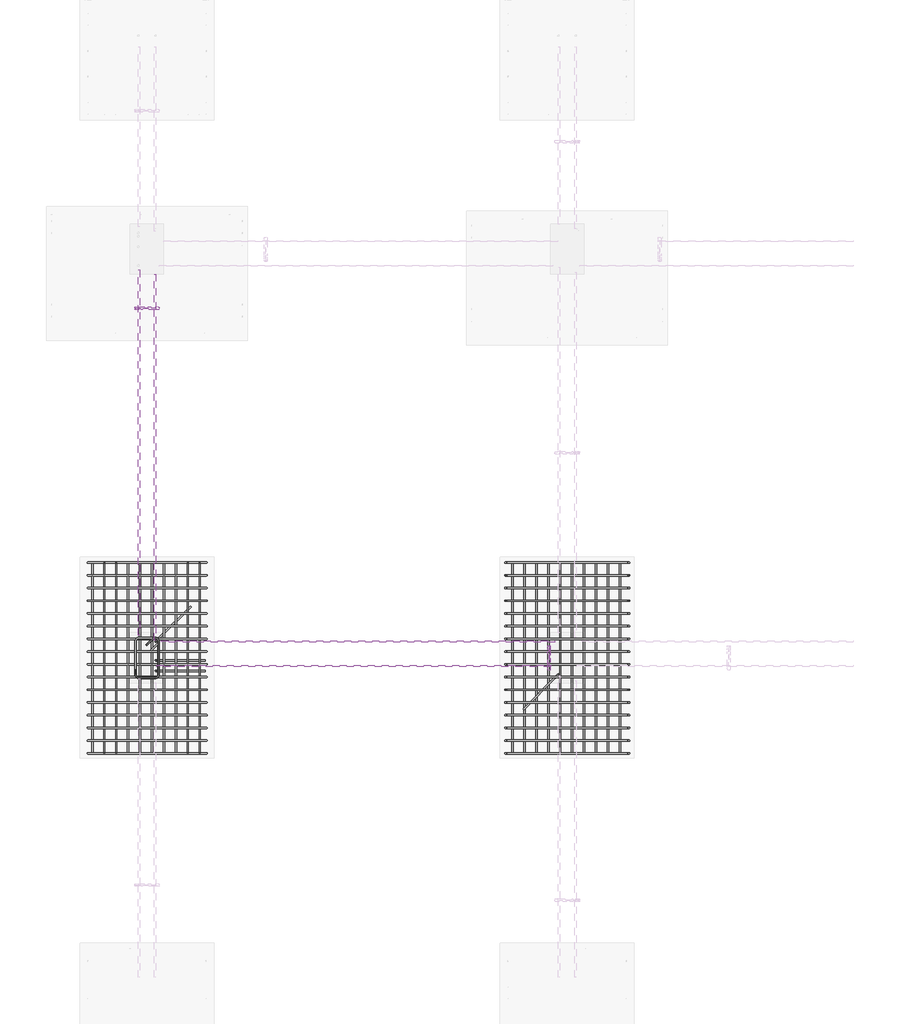
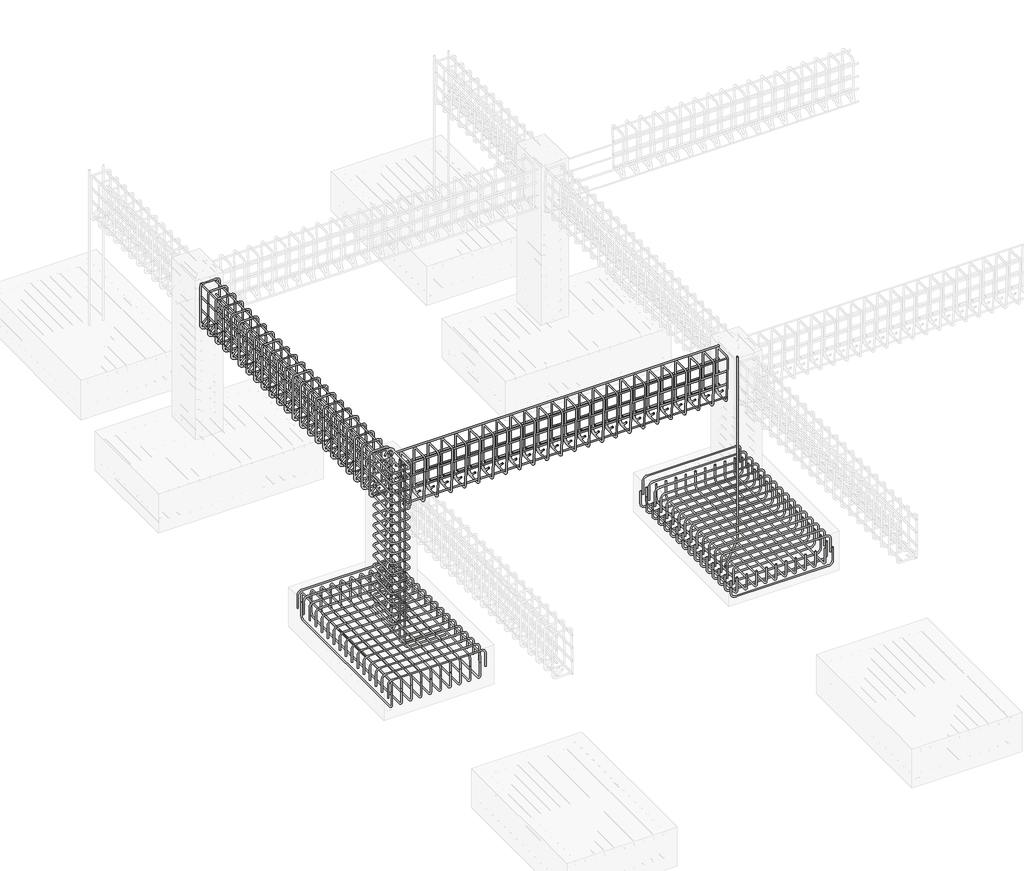
# One storey, part 4 of 20: 16 reinforcing bars.
"""IFC4 building model written with IfcOpenShell, lengths in millimetres."""

from ifc_helpers import new_model, si_unit, point, frame, origin, place, context, project, spatial, polyline, circle_curve, trimmed, segment, composite_curve, source, transform, mapped, element, save
from ifc_brep_helpers import swept_disk

model = new_model("IFC4")

# Units and contexts
model_context = context("Model", 3, world=origin())
ifc_project = project(units=[si_unit("LENGTHUNIT", "METRE", prefix="MILLI")], contexts=[model_context])

# Site, building, storey
site = spatial("IfcSite", under=ifc_project)
building = spatial("IfcBuilding", under=site)
storey = spatial("IfcBuildingStorey", under=building, Elevation=-1828.8)

# Reinforcing bars
placement = place(None, origin())
reinforcing_bar_shape = source(origin(), model_context, "Body", "SolidModel", [
    swept_disk(composite_curve([segment(polyline([(-6393.4168788, -1871.0168637, -2068.8), (-6393.4168788, -1871.0168637, -1921.5)]), True, "CONTINUOUS"), segment(trimmed(circle_curve(frame((-6347.0668788, -1871.0168637, -1921.5), z_axis=(0.0, 1.0, 0.0), x_axis=(-46.349999999999454, 0.0, 0.0)), 46.35), [point((-6393.4168788, -1871.0168637, -1921.5))], [point((-6347.0668788, -1871.0168637, -1875.15))], True, "CARTESIAN"), True, "CONTINUOUS"), segment(polyline([(-6347.0668788, -1871.0168637, -1875.15), (-5379.345487, -1871.0168637, -1875.15)]), True, "CONTINUOUS"), segment(trimmed(circle_curve(frame((-5379.345487, -1871.0168637, -1921.5), z_axis=(0.0, 1.0, 0.0), x_axis=(0.0, 0.0, 46.34999999999991)), 46.35), [point((-5379.345487, -1871.0168637, -1875.15))], [point((-5332.995487, -1871.0168637, -1921.5))], True, "CARTESIAN"), True, "CONTINUOUS"), segment(polyline([(-5332.995487, -1871.0168637, -1921.5), (-5332.995487, -1871.0168637, -2068.8)]), True, "CONTINUOUS")], self_intersect=False), 6.35),
])
element("IfcReinforcingBar", 1, at=placement, inside=storey, context=model_context, shape_type="MappedRepresentation", body=[
    mapped(reinforcing_bar_shape, transform((0.0, 0.0, 0.0), x_axis=(1.0, 0.0, 0.0), y_axis=(0.0, 1.0, 0.0), z_axis=(0.0, 0.0, 1.0))),
    mapped(reinforcing_bar_shape, transform((0.0, -113.82, 0.0), x_axis=(1.0, 0.0, 0.0), y_axis=(0.0, 1.0, 0.0), z_axis=(0.0, 0.0, 1.0))),
    mapped(reinforcing_bar_shape, transform((0.0, -227.64, 0.0), x_axis=(1.0, 0.0, 0.0), y_axis=(0.0, 1.0, 0.0), z_axis=(0.0, 0.0, 1.0))),
    mapped(reinforcing_bar_shape, transform((0.0, -341.46, 0.0), x_axis=(1.0, 0.0, 0.0), y_axis=(0.0, 1.0, 0.0), z_axis=(0.0, 0.0, 1.0))),
    mapped(reinforcing_bar_shape, transform((0.0, -455.28, 0.0), x_axis=(1.0, 0.0, 0.0), y_axis=(0.0, 1.0, 0.0), z_axis=(0.0, 0.0, 1.0))),
    mapped(reinforcing_bar_shape, transform((0.0, -569.1, 0.0), x_axis=(1.0, 0.0, 0.0), y_axis=(0.0, 1.0, 0.0), z_axis=(0.0, 0.0, 1.0))),
    mapped(reinforcing_bar_shape, transform((0.0, -682.92, 0.0), x_axis=(1.0, 0.0, 0.0), y_axis=(0.0, 1.0, 0.0), z_axis=(0.0, 0.0, 1.0))),
    mapped(reinforcing_bar_shape, transform((0.0, -796.74, 0.0), x_axis=(1.0, 0.0, 0.0), y_axis=(0.0, 1.0, 0.0), z_axis=(0.0, 0.0, 1.0))),
    mapped(reinforcing_bar_shape, transform((0.0, -910.56, 0.0), x_axis=(1.0, 0.0, 0.0), y_axis=(0.0, 1.0, 0.0), z_axis=(0.0, 0.0, 1.0))),
    mapped(reinforcing_bar_shape, transform((0.0, -1024.38, 0.0), x_axis=(1.0, 0.0, 0.0), y_axis=(0.0, 1.0, 0.0), z_axis=(0.0, 0.0, 1.0))),
    mapped(reinforcing_bar_shape, transform((0.0, -1138.2, 0.0), x_axis=(1.0, 0.0, 0.0), y_axis=(0.0, 1.0, 0.0), z_axis=(0.0, 0.0, 1.0))),
    mapped(reinforcing_bar_shape, transform((0.0, -1252.02, 0.0), x_axis=(1.0, 0.0, 0.0), y_axis=(0.0, 1.0, 0.0), z_axis=(0.0, 0.0, 1.0))),
    mapped(reinforcing_bar_shape, transform((0.0, -1365.84, 0.0), x_axis=(1.0, 0.0, 0.0), y_axis=(0.0, 1.0, 0.0), z_axis=(0.0, 0.0, 1.0))),
    mapped(reinforcing_bar_shape, transform((0.0, -1479.66, 0.0), x_axis=(1.0, 0.0, 0.0), y_axis=(0.0, 1.0, 0.0), z_axis=(0.0, 0.0, 1.0))),
    mapped(reinforcing_bar_shape, transform((0.0, -1593.48, 0.0), x_axis=(1.0, 0.0, 0.0), y_axis=(0.0, 1.0, 0.0), z_axis=(0.0, 0.0, 1.0))),
    mapped(reinforcing_bar_shape, transform((0.0, -1707.3, 0.0), x_axis=(1.0, 0.0, 0.0), y_axis=(0.0, 1.0, 0.0), z_axis=(0.0, 0.0, 1.0))),
])
reinforcing_bar_2_shape = source(origin(), model_context, "Body", "SolidModel", [
    swept_disk(composite_curve([segment(polyline([(-6353.8495286, -1871.0168637, -2008.6504502), (-6353.8495286, -1871.0168637, -2155.9504502)]), True, "CONTINUOUS"), segment(trimmed(circle_curve(frame((-6353.8495286, -1917.3668637, -2155.9504502), z_axis=(-1.0, 0.0, 0.0), x_axis=(0.0, 46.350000000000136, 0.0)), 46.35), [point((-6353.8495286, -1871.0168637, -2155.9504502))], [point((-6353.8495286, -1917.3668637, -2202.3004502))], True, "CARTESIAN"), True, "CONTINUOUS"), segment(polyline([(-6353.8495286, -1917.3668637, -2202.3004502), (-6353.8495286, -3531.9668637, -2202.3004502)]), True, "CONTINUOUS"), segment(trimmed(circle_curve(frame((-6353.8495286, -3531.9668637, -2155.9504502), z_axis=(-1.0, 0.0, 0.0), x_axis=(0.0, 0.0, -46.34999999999991)), 46.35), [point((-6353.8495286, -3531.9668637, -2202.3004502))], [point((-6353.8495286, -3578.3168637, -2155.9504502))], True, "CARTESIAN"), True, "CONTINUOUS"), segment(polyline([(-6353.8495286, -3578.3168637, -2155.9504502), (-6353.8495286, -3578.3168637, -2008.6504502)]), True, "CONTINUOUS")], self_intersect=False), 6.35),
])
element("IfcReinforcingBar", 2, at=placement, inside=storey, context=model_context, shape_type="MappedRepresentation", body=[
    mapped(reinforcing_bar_2_shape, transform((0.0, 0.0, 0.0), x_axis=(1.0, 0.0, 0.0), y_axis=(0.0, 1.0, 0.0), z_axis=(0.0, 0.0, 1.0))),
    mapped(reinforcing_bar_2_shape, transform((106.7711398, 0.0, 0.0), x_axis=(1.0, 0.0, 0.0), y_axis=(0.0, 1.0, 0.0), z_axis=(0.0, 0.0, 1.0))),
    mapped(reinforcing_bar_2_shape, transform((213.5422797, 0.0, 0.0), x_axis=(1.0, 0.0, 0.0), y_axis=(0.0, 1.0, 0.0), z_axis=(0.0, 0.0, 1.0))),
    mapped(reinforcing_bar_2_shape, transform((320.3134195, 0.0, 0.0), x_axis=(1.0, 0.0, 0.0), y_axis=(0.0, 1.0, 0.0), z_axis=(0.0, 0.0, 1.0))),
    mapped(reinforcing_bar_2_shape, transform((427.0845593, 0.0, 0.0), x_axis=(1.0, 0.0, 0.0), y_axis=(0.0, 1.0, 0.0), z_axis=(0.0, 0.0, 1.0))),
    mapped(reinforcing_bar_2_shape, transform((533.8556992, 0.0, 0.0), x_axis=(1.0, 0.0, 0.0), y_axis=(0.0, 1.0, 0.0), z_axis=(0.0, 0.0, 1.0))),
    mapped(reinforcing_bar_2_shape, transform((640.626839, 0.0, 0.0), x_axis=(1.0, 0.0, 0.0), y_axis=(0.0, 1.0, 0.0), z_axis=(0.0, 0.0, 1.0))),
    mapped(reinforcing_bar_2_shape, transform((747.3979788, 0.0, 0.0), x_axis=(1.0, 0.0, 0.0), y_axis=(0.0, 1.0, 0.0), z_axis=(0.0, 0.0, 1.0))),
    mapped(reinforcing_bar_2_shape, transform((854.1691187, 0.0, 0.0), x_axis=(1.0, 0.0, 0.0), y_axis=(0.0, 1.0, 0.0), z_axis=(0.0, 0.0, 1.0))),
    mapped(reinforcing_bar_2_shape, transform((960.9402585, 0.0, 0.0), x_axis=(1.0, 0.0, 0.0), y_axis=(0.0, 1.0, 0.0), z_axis=(0.0, 0.0, 1.0))),
])
reinforcing_bar_3_shape = source(origin(), model_context, "Body", "SolidModel", [
    swept_disk(composite_curve([segment(polyline([(-5392.9092701, -1871.0168637, -2088.5147466), (-5392.9092701, -1871.0168637, -1941.2147466)]), True, "CONTINUOUS"), segment(trimmed(circle_curve(frame((-5392.9092701, -1917.3668637, -1941.2147466), z_axis=(1.0, 0.0, 0.0), x_axis=(0.0, 46.350000000000136, 0.0)), 46.35), [point((-5392.9092701, -1871.0168637, -1941.2147466))], [point((-5392.9092701, -1917.3668637, -1894.8647466))], True, "CARTESIAN"), True, "CONTINUOUS"), segment(polyline([(-5392.9092701, -1917.3668637, -1894.8647466), (-5392.9092701, -3531.9668637, -1894.8647466)]), True, "CONTINUOUS"), segment(trimmed(circle_curve(frame((-5392.9092701, -3531.9668637, -1941.2147466), z_axis=(1.0, 0.0, 0.0), x_axis=(0.0, 0.0, 46.34999999999991)), 46.35), [point((-5392.9092701, -3531.9668637, -1894.8647466))], [point((-5392.9092701, -3578.3168637, -1941.2147466))], True, "CARTESIAN"), True, "CONTINUOUS"), segment(polyline([(-5392.9092701, -3578.3168637, -1941.2147466), (-5392.9092701, -3578.3168637, -2088.5147466)]), True, "CONTINUOUS")], self_intersect=False), 6.35),
])
element("IfcReinforcingBar", 3, at=placement, inside=storey, context=model_context, shape_type="MappedRepresentation", body=[
    mapped(reinforcing_bar_3_shape, transform((0.0, 0.0, 0.0), x_axis=(1.0, 0.0, 0.0), y_axis=(0.0, 1.0, 0.0), z_axis=(0.0, 0.0, 1.0))),
    mapped(reinforcing_bar_3_shape, transform((-106.7711398, 0.0, 0.0), x_axis=(1.0, 0.0, 0.0), y_axis=(0.0, 1.0, 0.0), z_axis=(0.0, 0.0, 1.0))),
    mapped(reinforcing_bar_3_shape, transform((-213.5422797, 0.0, 0.0), x_axis=(1.0, 0.0, 0.0), y_axis=(0.0, 1.0, 0.0), z_axis=(0.0, 0.0, 1.0))),
    mapped(reinforcing_bar_3_shape, transform((-320.3134195, 0.0, 0.0), x_axis=(1.0, 0.0, 0.0), y_axis=(0.0, 1.0, 0.0), z_axis=(0.0, 0.0, 1.0))),
    mapped(reinforcing_bar_3_shape, transform((-427.0845593, 0.0, 0.0), x_axis=(1.0, 0.0, 0.0), y_axis=(0.0, 1.0, 0.0), z_axis=(0.0, 0.0, 1.0))),
    mapped(reinforcing_bar_3_shape, transform((-533.8556992, 0.0, 0.0), x_axis=(1.0, 0.0, 0.0), y_axis=(0.0, 1.0, 0.0), z_axis=(0.0, 0.0, 1.0))),
    mapped(reinforcing_bar_3_shape, transform((-640.626839, 0.0, 0.0), x_axis=(1.0, 0.0, 0.0), y_axis=(0.0, 1.0, 0.0), z_axis=(0.0, 0.0, 1.0))),
    mapped(reinforcing_bar_3_shape, transform((-747.3979788, 0.0, 0.0), x_axis=(1.0, 0.0, 0.0), y_axis=(0.0, 1.0, 0.0), z_axis=(0.0, 0.0, 1.0))),
    mapped(reinforcing_bar_3_shape, transform((-854.1691187, 0.0, 0.0), x_axis=(1.0, 0.0, 0.0), y_axis=(0.0, 1.0, 0.0), z_axis=(0.0, 0.0, 1.0))),
    mapped(reinforcing_bar_3_shape, transform((-960.9402585, 0.0, 0.0), x_axis=(1.0, 0.0, 0.0), y_axis=(0.0, 1.0, 0.0), z_axis=(0.0, 0.0, 1.0))),
])
reinforcing_bar_4_shape = source(origin(), model_context, "Body", "SolidModel", [
    swept_disk(composite_curve([segment(polyline([(-1549.1360107, -1871.0168637, -2028.4704493), (-1549.1360107, -1871.0168637, -2175.7704493)]), True, "CONTINUOUS"), segment(trimmed(circle_curve(frame((-1595.4860107, -1871.0168637, -2175.7704493), z_axis=(0.0, 1.0, 0.0), x_axis=(46.34999999999991, 0.0, 0.0)), 46.35), [point((-1549.1360107, -1871.0168637, -2175.7704493))], [point((-1595.4860107, -1871.0168637, -2222.1204493))], True, "CARTESIAN"), True, "CONTINUOUS"), segment(polyline([(-1595.4860107, -1871.0168637, -2222.1204493), (-2610.0860107, -1871.0168637, -2222.1204493)]), True, "CONTINUOUS"), segment(trimmed(circle_curve(frame((-2610.0860107, -1871.0168637, -2175.7704493), z_axis=(0.0, 1.0, 0.0), x_axis=(0.0, 0.0, -46.34999999999991)), 46.35), [point((-2610.0860107, -1871.0168637, -2222.1204493))], [point((-2656.4360107, -1871.0168637, -2175.7704493))], True, "CARTESIAN"), True, "CONTINUOUS"), segment(polyline([(-2656.4360107, -1871.0168637, -2175.7704493), (-2656.4360107, -1871.0168637, -2028.4704493)]), True, "CONTINUOUS")], self_intersect=False), 6.35),
])
element("IfcReinforcingBar", 4, at=placement, inside=storey, context=model_context, shape_type="MappedRepresentation", body=[
    mapped(reinforcing_bar_4_shape, transform((0.0, 0.0, 0.0), x_axis=(1.0, 0.0, 0.0), y_axis=(0.0, 1.0, 0.0), z_axis=(0.0, 0.0, 1.0))),
    mapped(reinforcing_bar_4_shape, transform((0.0, -113.82, 0.0), x_axis=(1.0, 0.0, 0.0), y_axis=(0.0, 1.0, 0.0), z_axis=(0.0, 0.0, 1.0))),
    mapped(reinforcing_bar_4_shape, transform((0.0, -227.64, 0.0), x_axis=(1.0, 0.0, 0.0), y_axis=(0.0, 1.0, 0.0), z_axis=(0.0, 0.0, 1.0))),
    mapped(reinforcing_bar_4_shape, transform((0.0, -341.46, 0.0), x_axis=(1.0, 0.0, 0.0), y_axis=(0.0, 1.0, 0.0), z_axis=(0.0, 0.0, 1.0))),
    mapped(reinforcing_bar_4_shape, transform((0.0, -455.28, 0.0), x_axis=(1.0, 0.0, 0.0), y_axis=(0.0, 1.0, 0.0), z_axis=(0.0, 0.0, 1.0))),
    mapped(reinforcing_bar_4_shape, transform((0.0, -569.1, 0.0), x_axis=(1.0, 0.0, 0.0), y_axis=(0.0, 1.0, 0.0), z_axis=(0.0, 0.0, 1.0))),
    mapped(reinforcing_bar_4_shape, transform((0.0, -682.92, 0.0), x_axis=(1.0, 0.0, 0.0), y_axis=(0.0, 1.0, 0.0), z_axis=(0.0, 0.0, 1.0))),
    mapped(reinforcing_bar_4_shape, transform((0.0, -796.74, 0.0), x_axis=(1.0, 0.0, 0.0), y_axis=(0.0, 1.0, 0.0), z_axis=(0.0, 0.0, 1.0))),
    mapped(reinforcing_bar_4_shape, transform((0.0, -910.56, 0.0), x_axis=(1.0, 0.0, 0.0), y_axis=(0.0, 1.0, 0.0), z_axis=(0.0, 0.0, 1.0))),
    mapped(reinforcing_bar_4_shape, transform((0.0, -1024.38, 0.0), x_axis=(1.0, 0.0, 0.0), y_axis=(0.0, 1.0, 0.0), z_axis=(0.0, 0.0, 1.0))),
    mapped(reinforcing_bar_4_shape, transform((0.0, -1138.2, 0.0), x_axis=(1.0, 0.0, 0.0), y_axis=(0.0, 1.0, 0.0), z_axis=(0.0, 0.0, 1.0))),
    mapped(reinforcing_bar_4_shape, transform((0.0, -1252.02, 0.0), x_axis=(1.0, 0.0, 0.0), y_axis=(0.0, 1.0, 0.0), z_axis=(0.0, 0.0, 1.0))),
    mapped(reinforcing_bar_4_shape, transform((0.0, -1365.84, 0.0), x_axis=(1.0, 0.0, 0.0), y_axis=(0.0, 1.0, 0.0), z_axis=(0.0, 0.0, 1.0))),
    mapped(reinforcing_bar_4_shape, transform((0.0, -1479.66, 0.0), x_axis=(1.0, 0.0, 0.0), y_axis=(0.0, 1.0, 0.0), z_axis=(0.0, 0.0, 1.0))),
    mapped(reinforcing_bar_4_shape, transform((0.0, -1593.48, 0.0), x_axis=(1.0, 0.0, 0.0), y_axis=(0.0, 1.0, 0.0), z_axis=(0.0, 0.0, 1.0))),
    mapped(reinforcing_bar_4_shape, transform((0.0, -1707.3, 0.0), x_axis=(1.0, 0.0, 0.0), y_axis=(0.0, 1.0, 0.0), z_axis=(0.0, 0.0, 1.0))),
])
reinforcing_bar_5_shape = source(origin(), model_context, "Body", "SolidModel", [
    swept_disk(composite_curve([segment(polyline([(-2632.2616658, -1871.0168637, -2068.8), (-2632.2616658, -1871.0168637, -1921.5)]), True, "CONTINUOUS"), segment(trimmed(circle_curve(frame((-2585.9116658, -1871.0168637, -1921.5), z_axis=(0.0, 1.0, 0.0), x_axis=(-46.350000000000364, 0.0, 0.0)), 46.35), [point((-2632.2616658, -1871.0168637, -1921.5))], [point((-2585.9116658, -1871.0168637, -1875.15))], True, "CARTESIAN"), True, "CONTINUOUS"), segment(polyline([(-2585.9116658, -1871.0168637, -1875.15), (-1618.1902741, -1871.0168637, -1875.15)]), True, "CONTINUOUS"), segment(trimmed(circle_curve(frame((-1618.1902741, -1871.0168637, -1921.5), z_axis=(0.0, 1.0, 0.0), x_axis=(0.0, 0.0, 46.34999999999991)), 46.35), [point((-1618.1902741, -1871.0168637, -1875.15))], [point((-1571.8402741, -1871.0168637, -1921.5))], True, "CARTESIAN"), True, "CONTINUOUS"), segment(polyline([(-1571.8402741, -1871.0168637, -1921.5), (-1571.8402741, -1871.0168637, -2068.8)]), True, "CONTINUOUS")], self_intersect=False), 6.35),
])
element("IfcReinforcingBar", 5, at=placement, inside=storey, context=model_context, shape_type="MappedRepresentation", body=[
    mapped(reinforcing_bar_5_shape, transform((0.0, 0.0, 0.0), x_axis=(1.0, 0.0, 0.0), y_axis=(0.0, 1.0, 0.0), z_axis=(0.0, 0.0, 1.0))),
    mapped(reinforcing_bar_5_shape, transform((0.0, -113.82, 0.0), x_axis=(1.0, 0.0, 0.0), y_axis=(0.0, 1.0, 0.0), z_axis=(0.0, 0.0, 1.0))),
    mapped(reinforcing_bar_5_shape, transform((0.0, -227.64, 0.0), x_axis=(1.0, 0.0, 0.0), y_axis=(0.0, 1.0, 0.0), z_axis=(0.0, 0.0, 1.0))),
    mapped(reinforcing_bar_5_shape, transform((0.0, -341.46, 0.0), x_axis=(1.0, 0.0, 0.0), y_axis=(0.0, 1.0, 0.0), z_axis=(0.0, 0.0, 1.0))),
    mapped(reinforcing_bar_5_shape, transform((0.0, -455.28, 0.0), x_axis=(1.0, 0.0, 0.0), y_axis=(0.0, 1.0, 0.0), z_axis=(0.0, 0.0, 1.0))),
    mapped(reinforcing_bar_5_shape, transform((0.0, -569.1, 0.0), x_axis=(1.0, 0.0, 0.0), y_axis=(0.0, 1.0, 0.0), z_axis=(0.0, 0.0, 1.0))),
    mapped(reinforcing_bar_5_shape, transform((0.0, -682.92, 0.0), x_axis=(1.0, 0.0, 0.0), y_axis=(0.0, 1.0, 0.0), z_axis=(0.0, 0.0, 1.0))),
    mapped(reinforcing_bar_5_shape, transform((0.0, -796.74, 0.0), x_axis=(1.0, 0.0, 0.0), y_axis=(0.0, 1.0, 0.0), z_axis=(0.0, 0.0, 1.0))),
    mapped(reinforcing_bar_5_shape, transform((0.0, -910.56, 0.0), x_axis=(1.0, 0.0, 0.0), y_axis=(0.0, 1.0, 0.0), z_axis=(0.0, 0.0, 1.0))),
    mapped(reinforcing_bar_5_shape, transform((0.0, -1024.38, 0.0), x_axis=(1.0, 0.0, 0.0), y_axis=(0.0, 1.0, 0.0), z_axis=(0.0, 0.0, 1.0))),
    mapped(reinforcing_bar_5_shape, transform((0.0, -1138.2, 0.0), x_axis=(1.0, 0.0, 0.0), y_axis=(0.0, 1.0, 0.0), z_axis=(0.0, 0.0, 1.0))),
    mapped(reinforcing_bar_5_shape, transform((0.0, -1252.02, 0.0), x_axis=(1.0, 0.0, 0.0), y_axis=(0.0, 1.0, 0.0), z_axis=(0.0, 0.0, 1.0))),
    mapped(reinforcing_bar_5_shape, transform((0.0, -1365.84, 0.0), x_axis=(1.0, 0.0, 0.0), y_axis=(0.0, 1.0, 0.0), z_axis=(0.0, 0.0, 1.0))),
    mapped(reinforcing_bar_5_shape, transform((0.0, -1479.66, 0.0), x_axis=(1.0, 0.0, 0.0), y_axis=(0.0, 1.0, 0.0), z_axis=(0.0, 0.0, 1.0))),
    mapped(reinforcing_bar_5_shape, transform((0.0, -1593.48, 0.0), x_axis=(1.0, 0.0, 0.0), y_axis=(0.0, 1.0, 0.0), z_axis=(0.0, 0.0, 1.0))),
    mapped(reinforcing_bar_5_shape, transform((0.0, -1707.3, 0.0), x_axis=(1.0, 0.0, 0.0), y_axis=(0.0, 1.0, 0.0), z_axis=(0.0, 0.0, 1.0))),
])
reinforcing_bar_6_shape = source(origin(), model_context, "Body", "SolidModel", [
    swept_disk(composite_curve([segment(polyline([(-2592.6943156, -1871.0168637, -2008.6504502), (-2592.6943156, -1871.0168637, -2155.9504502)]), True, "CONTINUOUS"), segment(trimmed(circle_curve(frame((-2592.6943156, -1917.3668637, -2155.9504502), z_axis=(-1.0, 0.0, 0.0), x_axis=(0.0, 46.350000000000136, 0.0)), 46.35), [point((-2592.6943156, -1871.0168637, -2155.9504502))], [point((-2592.6943156, -1917.3668637, -2202.3004502))], True, "CARTESIAN"), True, "CONTINUOUS"), segment(polyline([(-2592.6943156, -1917.3668637, -2202.3004502), (-2592.6943156, -3531.9668637, -2202.3004502)]), True, "CONTINUOUS"), segment(trimmed(circle_curve(frame((-2592.6943156, -3531.9668637, -2155.9504502), z_axis=(-1.0, 0.0, 0.0), x_axis=(0.0, 0.0, -46.34999999999991)), 46.35), [point((-2592.6943156, -3531.9668637, -2202.3004502))], [point((-2592.6943156, -3578.3168637, -2155.9504502))], True, "CARTESIAN"), True, "CONTINUOUS"), segment(polyline([(-2592.6943156, -3578.3168637, -2155.9504502), (-2592.6943156, -3578.3168637, -2008.6504502)]), True, "CONTINUOUS")], self_intersect=False), 6.35),
])
element("IfcReinforcingBar", 6, at=placement, inside=storey, context=model_context, shape_type="MappedRepresentation", body=[
    mapped(reinforcing_bar_6_shape, transform((0.0, 0.0, 0.0), x_axis=(1.0, 0.0, 0.0), y_axis=(0.0, 1.0, 0.0), z_axis=(0.0, 0.0, 1.0))),
    mapped(reinforcing_bar_6_shape, transform((106.7711398, 0.0, 0.0), x_axis=(1.0, 0.0, 0.0), y_axis=(0.0, 1.0, 0.0), z_axis=(0.0, 0.0, 1.0))),
    mapped(reinforcing_bar_6_shape, transform((213.5422797, 0.0, 0.0), x_axis=(1.0, 0.0, 0.0), y_axis=(0.0, 1.0, 0.0), z_axis=(0.0, 0.0, 1.0))),
    mapped(reinforcing_bar_6_shape, transform((320.3134195, 0.0, 0.0), x_axis=(1.0, 0.0, 0.0), y_axis=(0.0, 1.0, 0.0), z_axis=(0.0, 0.0, 1.0))),
    mapped(reinforcing_bar_6_shape, transform((427.0845593, 0.0, 0.0), x_axis=(1.0, 0.0, 0.0), y_axis=(0.0, 1.0, 0.0), z_axis=(0.0, 0.0, 1.0))),
    mapped(reinforcing_bar_6_shape, transform((533.8556992, 0.0, 0.0), x_axis=(1.0, 0.0, 0.0), y_axis=(0.0, 1.0, 0.0), z_axis=(0.0, 0.0, 1.0))),
    mapped(reinforcing_bar_6_shape, transform((640.626839, 0.0, 0.0), x_axis=(1.0, 0.0, 0.0), y_axis=(0.0, 1.0, 0.0), z_axis=(0.0, 0.0, 1.0))),
    mapped(reinforcing_bar_6_shape, transform((747.3979788, 0.0, 0.0), x_axis=(1.0, 0.0, 0.0), y_axis=(0.0, 1.0, 0.0), z_axis=(0.0, 0.0, 1.0))),
    mapped(reinforcing_bar_6_shape, transform((854.1691187, 0.0, 0.0), x_axis=(1.0, 0.0, 0.0), y_axis=(0.0, 1.0, 0.0), z_axis=(0.0, 0.0, 1.0))),
    mapped(reinforcing_bar_6_shape, transform((960.9402585, 0.0, 0.0), x_axis=(1.0, 0.0, 0.0), y_axis=(0.0, 1.0, 0.0), z_axis=(0.0, 0.0, 1.0))),
])
reinforcing_bar_7_shape = source(origin(), model_context, "Body", "SolidModel", [
    swept_disk(composite_curve([segment(polyline([(-5869.5525842, -2610.942629, -46.35), (-5813.8090212, -2555.1990661, -46.35)]), True, "CONTINUOUS"), segment(trimmed(circle_curve(frame((-5791.6412236, -2577.3668637, -46.35), z_axis=(0.0, 0.0, -1.0), x_axis=(-22.167797600000085, 22.167797600000085, 0.0)), 31.35), [point((-5813.8090212, -2555.1990661, -46.35))], [point((-5760.2912236, -2577.3668637, -46.35))], True, "CARTESIAN"), True, "CONTINUOUS"), segment(polyline([(-5760.2912236, -2577.3668637, -46.35), (-5760.2912236, -2871.9668637, -46.35)]), True, "CONTINUOUS"), segment(trimmed(circle_curve(frame((-5791.6412236, -2871.9668637, -46.35), z_axis=(0.0, 0.0, -1.0), x_axis=(31.349999999999454, 0.0, 0.0)), 31.35), [point((-5760.2912236, -2871.9668637, -46.35))], [point((-5791.6412236, -2903.3168637, -46.35))], True, "CARTESIAN"), True, "CONTINUOUS"), segment(polyline([(-5791.6412236, -2903.3168637, -46.35), (-5936.2412236, -2903.3168637, -46.35)]), True, "CONTINUOUS"), segment(trimmed(circle_curve(frame((-5936.2412236, -2871.9866488, -45.2363875), z_axis=(0.0, 0.035521928334481916, -0.9993688971583016), x_axis=(0.0, -31.3302149000001, -1.1136125000000021)), 31.35), [point((-5936.2412236, -2903.3168637, -46.35))], [point((-5967.5912236, -2871.9866488, -45.2363875))], True, "CARTESIAN"), True, "CONTINUOUS"), segment(polyline([(-5967.5912236, -2871.9866488, -45.2363875), (-5967.5912236, -2577.3470786, -34.7636125)]), True, "CONTINUOUS"), segment(trimmed(circle_curve(frame((-5936.2412236, -2577.3470786, -34.7636125), z_axis=(0.0, 0.035521928334481916, -0.9993688971583016), x_axis=(-31.350000000000364, 0.0, 0.0)), 31.35), [point((-5967.5912236, -2577.3470786, -34.7636125))], [point((-5936.2412236, -2546.0168637, -33.65))], True, "CARTESIAN"), True, "CONTINUOUS"), segment(polyline([(-5936.2412236, -2546.0168637, -33.65), (-5791.6412236, -2546.0168637, -33.65)]), True, "CONTINUOUS"), segment(trimmed(circle_curve(frame((-5791.6412236, -2577.3668637, -33.65), z_axis=(0.0, 0.0, -1.0), x_axis=(0.0, 31.34999999999991, 0.0)), 31.35), [point((-5791.6412236, -2546.0168637, -33.65))], [point((-5769.473426, -2599.5346613, -33.65))], True, "CARTESIAN"), True, "CONTINUOUS"), segment(polyline([(-5769.473426, -2599.5346613, -33.65), (-5825.216989, -2655.2782242, -33.65)]), True, "CONTINUOUS")], self_intersect=False), 6.35),
])
element("IfcReinforcingBar", 7, at=placement, inside=storey, context=model_context, shape_type="MappedRepresentation", body=[
    mapped(reinforcing_bar_7_shape, transform((0.0, 0.0, 0.0), x_axis=(1.0, 0.0, 0.0), y_axis=(0.0, 1.0, 0.0), z_axis=(0.0, 0.0, 1.0))),
    mapped(reinforcing_bar_7_shape, transform((0.0, 0.0, -115.74), x_axis=(1.0, 0.0, 0.0), y_axis=(0.0, 1.0, 0.0), z_axis=(0.0, 0.0, 1.0))),
    mapped(reinforcing_bar_7_shape, transform((0.0, 0.0, -231.48), x_axis=(1.0, 0.0, 0.0), y_axis=(0.0, 1.0, 0.0), z_axis=(0.0, 0.0, 1.0))),
    mapped(reinforcing_bar_7_shape, transform((0.0, 0.0, -347.22), x_axis=(1.0, 0.0, 0.0), y_axis=(0.0, 1.0, 0.0), z_axis=(0.0, 0.0, 1.0))),
    mapped(reinforcing_bar_7_shape, transform((0.0, 0.0, -462.96), x_axis=(1.0, 0.0, 0.0), y_axis=(0.0, 1.0, 0.0), z_axis=(0.0, 0.0, 1.0))),
    mapped(reinforcing_bar_7_shape, transform((0.0, 0.0, -578.7), x_axis=(1.0, 0.0, 0.0), y_axis=(0.0, 1.0, 0.0), z_axis=(0.0, 0.0, 1.0))),
    mapped(reinforcing_bar_7_shape, transform((0.0, 0.0, -694.44), x_axis=(1.0, 0.0, 0.0), y_axis=(0.0, 1.0, 0.0), z_axis=(0.0, 0.0, 1.0))),
    mapped(reinforcing_bar_7_shape, transform((0.0, 0.0, -810.18), x_axis=(1.0, 0.0, 0.0), y_axis=(0.0, 1.0, 0.0), z_axis=(0.0, 0.0, 1.0))),
    mapped(reinforcing_bar_7_shape, transform((0.0, 0.0, -925.92), x_axis=(1.0, 0.0, 0.0), y_axis=(0.0, 1.0, 0.0), z_axis=(0.0, 0.0, 1.0))),
    mapped(reinforcing_bar_7_shape, transform((0.0, 0.0, -1041.66), x_axis=(1.0, 0.0, 0.0), y_axis=(0.0, 1.0, 0.0), z_axis=(0.0, 0.0, 1.0))),
    mapped(reinforcing_bar_7_shape, transform((0.0, 0.0, -1157.4), x_axis=(1.0, 0.0, 0.0), y_axis=(0.0, 1.0, 0.0), z_axis=(0.0, 0.0, 1.0))),
    mapped(reinforcing_bar_7_shape, transform((0.0, 0.0, -1273.14), x_axis=(1.0, 0.0, 0.0), y_axis=(0.0, 1.0, 0.0), z_axis=(0.0, 0.0, 1.0))),
    mapped(reinforcing_bar_7_shape, transform((0.0, 0.0, -1388.88), x_axis=(1.0, 0.0, 0.0), y_axis=(0.0, 1.0, 0.0), z_axis=(0.0, 0.0, 1.0))),
    mapped(reinforcing_bar_7_shape, transform((0.0, 0.0, -1504.62), x_axis=(1.0, 0.0, 0.0), y_axis=(0.0, 1.0, 0.0), z_axis=(0.0, 0.0, 1.0))),
    mapped(reinforcing_bar_7_shape, transform((0.0, 0.0, -1620.36), x_axis=(1.0, 0.0, 0.0), y_axis=(0.0, 1.0, 0.0), z_axis=(0.0, 0.0, 1.0))),
    mapped(reinforcing_bar_7_shape, transform((0.0, 0.0, -1736.1), x_axis=(1.0, 0.0, 0.0), y_axis=(0.0, 1.0, 0.0), z_axis=(0.0, 0.0, 1.0))),
])
element("IfcReinforcingBar", 8, at=placement, inside=storey, context=model_context, shape_type="SolidModel", body=[
    swept_disk(composite_curve([segment(polyline([(-5473.271622, -2265.1629186, -2151.8747939), (-5754.0052693, -2545.8965659, -2151.8747939)]), True, "CONTINUOUS"), segment(trimmed(circle_curve(frame((-5754.0052693, -2545.8965659, -2105.5247939), z_axis=(-0.7071067811865442, 0.7071067811865509, 0.0), x_axis=(0.0, 0.0, -46.34999999999991)), 46.35), [point((-5754.0052693, -2545.8965659, -2151.8747939))], [point((-5786.7796686, -2578.6709652, -2105.5247939))], True, "CARTESIAN"), True, "CONTINUOUS"), segment(polyline([(-5786.7796686, -2578.6709652, -2105.5247939), (-5786.7796686, -2578.6709652, -40.0)]), True, "CONTINUOUS")], self_intersect=False), 6.35),
])
reinforcing_bar_8_shape = source(origin(), model_context, "Body", "SolidModel", [
    swept_disk(composite_curve([segment(polyline([(-5343.4123372, -2745.9908411, -2151.8747939), (-5740.4296686, -2745.9908411, -2151.8747939)]), True, "CONTINUOUS"), segment(trimmed(circle_curve(frame((-5740.4296686, -2745.9908411, -2105.5247939), z_axis=(0.0, 1.0, 0.0), x_axis=(0.0, 0.0, -46.34999999999991)), 46.35), [point((-5740.4296686, -2745.9908411, -2151.8747939))], [point((-5786.7796686, -2745.9908411, -2105.5247939))], True, "CARTESIAN"), True, "CONTINUOUS"), segment(polyline([(-5786.7796686, -2745.9908411, -2105.5247939), (-5786.7796686, -2745.9908411, -40.0)]), True, "CONTINUOUS")], self_intersect=False), 6.35),
])
element("IfcReinforcingBar", 9, at=placement, inside=storey, context=model_context, shape_type="MappedRepresentation", body=[
    mapped(reinforcing_bar_8_shape, transform((0.0, 0.0, 0.0), x_axis=(1.0, 0.0, 0.0), y_axis=(0.0, 1.0, 0.0), z_axis=(0.0, 0.0, 1.0))),
    mapped(reinforcing_bar_8_shape, transform((0.0, -93.9182821, 0.0), x_axis=(1.0, 0.0, 0.0), y_axis=(0.0, 1.0, 0.0), z_axis=(0.0, 0.0, 1.0))),
])
element("IfcReinforcingBar", 10, at=placement, inside=storey, context=model_context, shape_type="SolidModel", body=[
    swept_disk(composite_curve([segment(polyline([(-2493.4556123, -3184.1708088, -2151.8747939), (-2212.721965, -2903.4371615, -2151.8747939)]), True, "CONTINUOUS"), segment(trimmed(circle_curve(frame((-2212.721965, -2903.4371615, -2105.5247939), z_axis=(0.7071067811865442, -0.7071067811865509, 0.0), x_axis=(0.0, 0.0, -46.34999999999991)), 46.35), [point((-2212.721965, -2903.4371615, -2151.8747939))], [point((-2179.9475657, -2870.6627622, -2105.5247939))], True, "CARTESIAN"), True, "CONTINUOUS"), segment(polyline([(-2179.9475657, -2870.6627622, -2105.5247939), (-2179.9475657, -2870.6627622, -40.0)]), True, "CONTINUOUS")], self_intersect=False), 6.35),
])
reinforcing_bar_9_shape = source(origin(), model_context, "Body", "SolidModel", [
    swept_disk(composite_curve([segment(polyline([(-5858.3298631, -2493.3168637, -488.7242346), (-5914.073426, -2493.3168637, -544.4677976)]), True, "CONTINUOUS"), segment(trimmed(circle_curve(frame((-5936.2412236, -2493.3168637, -522.3), z_axis=(0.0, 1.0, 0.0), x_axis=(22.167797600000085, 0.0, -22.167797600000085)), 31.35), [point((-5914.073426, -2493.3168637, -544.4677976))], [point((-5967.5912236, -2493.3168637, -522.3))], True, "CARTESIAN"), True, "CONTINUOUS"), segment(polyline([(-5967.5912236, -2493.3168637, -522.3), (-5967.5912236, -2493.3168637, -77.7)]), True, "CONTINUOUS"), segment(trimmed(circle_curve(frame((-5936.2412236, -2493.3168637, -77.7), z_axis=(0.0, 1.0, 0.0), x_axis=(-31.350000000000364, 0.0, 0.0)), 31.35), [point((-5967.5912236, -2493.3168637, -77.7))], [point((-5936.2412236, -2493.3168637, -46.35))], True, "CARTESIAN"), True, "CONTINUOUS"), segment(polyline([(-5936.2412236, -2493.3168637, -46.35), (-5791.6412236, -2493.3168637, -46.35)]), True, "CONTINUOUS"), segment(trimmed(circle_curve(frame((-5791.6412236, -2494.1014493, -77.6901807), z_axis=(0.0, 0.9996867842138424, -0.025026655153786322), x_axis=(0.0, 0.7845855999999003, 31.340180699999998)), 31.35), [point((-5791.6412236, -2493.3168637, -46.35))], [point((-5760.2912236, -2494.1014493, -77.6901807))], True, "CARTESIAN"), True, "CONTINUOUS"), segment(polyline([(-5760.2912236, -2494.1014493, -77.6901807), (-5760.2912236, -2505.232278, -522.3098193)]), True, "CONTINUOUS"), segment(trimmed(circle_curve(frame((-5791.6412236, -2505.232278, -522.3098193), z_axis=(0.0, 0.9996867842138424, -0.025026655153786322), x_axis=(31.349999999999454, 0.0, 0.0)), 31.35), [point((-5760.2912236, -2505.232278, -522.3098193))], [point((-5791.6412236, -2506.0168637, -553.65))], True, "CARTESIAN"), True, "CONTINUOUS"), segment(polyline([(-5791.6412236, -2506.0168637, -553.65), (-5936.2412236, -2506.0168637, -553.65)]), True, "CONTINUOUS"), segment(trimmed(circle_curve(frame((-5936.2412236, -2506.0168637, -522.3), z_axis=(0.0, 1.0, 0.0), x_axis=(0.0, 0.0, -31.350000000000023)), 31.35), [point((-5936.2412236, -2506.0168637, -553.65))], [point((-5958.4090212, -2506.0168637, -500.1322024))], True, "CARTESIAN"), True, "CONTINUOUS"), segment(polyline([(-5958.4090212, -2506.0168637, -500.1322024), (-5902.6654583, -2506.0168637, -444.3886395)]), True, "CONTINUOUS")], self_intersect=False), 6.35),
])
element("IfcReinforcingBar", 11, at=placement, inside=storey, context=model_context, shape_type="MappedRepresentation", body=[
    mapped(reinforcing_bar_9_shape, transform((0.0, 0.0, 0.0), x_axis=(1.0, 0.0, 0.0), y_axis=(0.0, 1.0, 0.0), z_axis=(0.0, 0.0, 1.0))),
    mapped(reinforcing_bar_9_shape, transform((0.0, 145.2227273, 0.0), x_axis=(1.0, 0.0, 0.0), y_axis=(0.0, 1.0, 0.0), z_axis=(0.0, 0.0, 1.0))),
    mapped(reinforcing_bar_9_shape, transform((0.0, 290.4454545, 0.0), x_axis=(1.0, 0.0, 0.0), y_axis=(0.0, 1.0, 0.0), z_axis=(0.0, 0.0, 1.0))),
    mapped(reinforcing_bar_9_shape, transform((0.0, 435.6681818, 0.0), x_axis=(1.0, 0.0, 0.0), y_axis=(0.0, 1.0, 0.0), z_axis=(0.0, 0.0, 1.0))),
    mapped(reinforcing_bar_9_shape, transform((0.0, 580.8909091, 0.0), x_axis=(1.0, 0.0, 0.0), y_axis=(0.0, 1.0, 0.0), z_axis=(0.0, 0.0, 1.0))),
    mapped(reinforcing_bar_9_shape, transform((0.0, 726.1136364, 0.0), x_axis=(1.0, 0.0, 0.0), y_axis=(0.0, 1.0, 0.0), z_axis=(0.0, 0.0, 1.0))),
    mapped(reinforcing_bar_9_shape, transform((0.0, 871.3363636, 0.0), x_axis=(1.0, 0.0, 0.0), y_axis=(0.0, 1.0, 0.0), z_axis=(0.0, 0.0, 1.0))),
    mapped(reinforcing_bar_9_shape, transform((0.0, 1016.5590909, 0.0), x_axis=(1.0, 0.0, 0.0), y_axis=(0.0, 1.0, 0.0), z_axis=(0.0, 0.0, 1.0))),
    mapped(reinforcing_bar_9_shape, transform((0.0, 1161.7818182, 0.0), x_axis=(1.0, 0.0, 0.0), y_axis=(0.0, 1.0, 0.0), z_axis=(0.0, 0.0, 1.0))),
    mapped(reinforcing_bar_9_shape, transform((0.0, 1307.0045455, 0.0), x_axis=(1.0, 0.0, 0.0), y_axis=(0.0, 1.0, 0.0), z_axis=(0.0, 0.0, 1.0))),
    mapped(reinforcing_bar_9_shape, transform((0.0, 1452.2272727, 0.0), x_axis=(1.0, 0.0, 0.0), y_axis=(0.0, 1.0, 0.0), z_axis=(0.0, 0.0, 1.0))),
    mapped(reinforcing_bar_9_shape, transform((0.0, 1597.45, 0.0), x_axis=(1.0, 0.0, 0.0), y_axis=(0.0, 1.0, 0.0), z_axis=(0.0, 0.0, 1.0))),
    mapped(reinforcing_bar_9_shape, transform((0.0, 1742.6727273, 0.0), x_axis=(1.0, 0.0, 0.0), y_axis=(0.0, 1.0, 0.0), z_axis=(0.0, 0.0, 1.0))),
    mapped(reinforcing_bar_9_shape, transform((0.0, 1887.8954545, 0.0), x_axis=(1.0, 0.0, 0.0), y_axis=(0.0, 1.0, 0.0), z_axis=(0.0, 0.0, 1.0))),
    mapped(reinforcing_bar_9_shape, transform((0.0, 2033.1181818, 0.0), x_axis=(1.0, 0.0, 0.0), y_axis=(0.0, 1.0, 0.0), z_axis=(0.0, 0.0, 1.0))),
    mapped(reinforcing_bar_9_shape, transform((0.0, 2178.3409091, 0.0), x_axis=(1.0, 0.0, 0.0), y_axis=(0.0, 1.0, 0.0), z_axis=(0.0, 0.0, 1.0))),
    mapped(reinforcing_bar_9_shape, transform((0.0, 2323.5636364, 0.0), x_axis=(1.0, 0.0, 0.0), y_axis=(0.0, 1.0, 0.0), z_axis=(0.0, 0.0, 1.0))),
    mapped(reinforcing_bar_9_shape, transform((0.0, 2468.7863636, 0.0), x_axis=(1.0, 0.0, 0.0), y_axis=(0.0, 1.0, 0.0), z_axis=(0.0, 0.0, 1.0))),
    mapped(reinforcing_bar_9_shape, transform((0.0, 2614.0090909, 0.0), x_axis=(1.0, 0.0, 0.0), y_axis=(0.0, 1.0, 0.0), z_axis=(0.0, 0.0, 1.0))),
    mapped(reinforcing_bar_9_shape, transform((0.0, 2759.2318182, 0.0), x_axis=(1.0, 0.0, 0.0), y_axis=(0.0, 1.0, 0.0), z_axis=(0.0, 0.0, 1.0))),
    mapped(reinforcing_bar_9_shape, transform((0.0, 2904.4545455, 0.0), x_axis=(1.0, 0.0, 0.0), y_axis=(0.0, 1.0, 0.0), z_axis=(0.0, 0.0, 1.0))),
    mapped(reinforcing_bar_9_shape, transform((0.0, 3049.6772727, 0.0), x_axis=(1.0, 0.0, 0.0), y_axis=(0.0, 1.0, 0.0), z_axis=(0.0, 0.0, 1.0))),
    mapped(reinforcing_bar_9_shape, transform((0.0, 3194.9, 0.0), x_axis=(1.0, 0.0, 0.0), y_axis=(0.0, 1.0, 0.0), z_axis=(0.0, 0.0, 1.0))),
])
reinforcing_bar_10_shape = source(origin(), model_context, "Body", "SolidModel", [
    swept_disk(composite_curve([segment(polyline([(-5936.2412236, -2520.7202711, -522.0844), (-5936.2412236, 747.9331363, -522.0844)]), True, "CONTINUOUS")], self_intersect=False), 6.35),
])
element("IfcReinforcingBar", 12, at=placement, inside=storey, context=model_context, shape_type="MappedRepresentation", body=[
    mapped(reinforcing_bar_10_shape, transform((0.0, 0.0, 0.0), x_axis=(1.0, 0.0, 0.0), y_axis=(0.0, 1.0, 0.0), z_axis=(0.0, 0.0, 1.0))),
    mapped(reinforcing_bar_10_shape, transform((0.0, 0.0, 147.799393), x_axis=(1.0, 0.0, 0.0), y_axis=(0.0, 1.0, 0.0), z_axis=(0.0, 0.0, 1.0))),
    mapped(reinforcing_bar_10_shape, transform((0.0, 0.0, 295.598786), x_axis=(1.0, 0.0, 0.0), y_axis=(0.0, 1.0, 0.0), z_axis=(0.0, 0.0, 1.0))),
    mapped(reinforcing_bar_10_shape, transform((0.0, 0.0, 443.398179), x_axis=(1.0, 0.0, 0.0), y_axis=(0.0, 1.0, 0.0), z_axis=(0.0, 0.0, 1.0))),
])
reinforcing_bar_11_shape = source(origin(), model_context, "Body", "SolidModel", [
    swept_disk(composite_curve([segment(polyline([(-5791.6412236, -2564.7737816, -522.0844), (-5791.6412236, 709.1189279, -522.0844)]), True, "CONTINUOUS")], self_intersect=False), 6.35),
])
element("IfcReinforcingBar", 13, at=placement, inside=storey, context=model_context, shape_type="MappedRepresentation", body=[
    mapped(reinforcing_bar_11_shape, transform((0.0, 0.0, 0.0), x_axis=(1.0, 0.0, 0.0), y_axis=(0.0, 1.0, 0.0), z_axis=(0.0, 0.0, 1.0))),
    mapped(reinforcing_bar_11_shape, transform((0.0, 0.0, 147.799393), x_axis=(1.0, 0.0, 0.0), y_axis=(0.0, 1.0, 0.0), z_axis=(0.0, 0.0, 1.0))),
    mapped(reinforcing_bar_11_shape, transform((0.0, 0.0, 295.598786), x_axis=(1.0, 0.0, 0.0), y_axis=(0.0, 1.0, 0.0), z_axis=(0.0, 0.0, 1.0))),
    mapped(reinforcing_bar_11_shape, transform((0.0, 0.0, 443.398179), x_axis=(1.0, 0.0, 0.0), y_axis=(0.0, 1.0, 0.0), z_axis=(0.0, 0.0, 1.0))),
])
reinforcing_bar_12_shape = source(origin(), model_context, "Body", "SolidModel", [
    swept_disk(composite_curve([segment(polyline([(-5707.5912236, -2730.2782242, -488.7242346), (-5707.5912236, -2674.5346613, -544.4677976)]), True, "CONTINUOUS"), segment(trimmed(circle_curve(frame((-5707.5912236, -2652.3668637, -522.3), z_axis=(1.0, 0.0, 0.0), x_axis=(0.0, -22.167797600000085, -22.167797600000085)), 31.35), [point((-5707.5912236, -2674.5346613, -544.4677976))], [point((-5707.5912236, -2621.0168637, -522.3))], True, "CARTESIAN"), True, "CONTINUOUS"), segment(polyline([(-5707.5912236, -2621.0168637, -522.3), (-5707.5912236, -2621.0168637, -77.7)]), True, "CONTINUOUS"), segment(trimmed(circle_curve(frame((-5707.5912236, -2652.3668637, -77.7), z_axis=(1.0, 0.0, 0.0), x_axis=(0.0, 31.34999999999991, 0.0)), 31.35), [point((-5707.5912236, -2621.0168637, -77.7))], [point((-5707.5912236, -2652.3668637, -46.35))], True, "CARTESIAN"), True, "CONTINUOUS"), segment(polyline([(-5707.5912236, -2652.3668637, -46.35), (-5707.5912236, -2796.9668637, -46.35)]), True, "CONTINUOUS"), segment(trimmed(circle_curve(frame((-5708.3758093, -2796.9668637, -77.6901807), z_axis=(0.9996867842138424, 0.0, -0.025026655153786322), x_axis=(0.7845856999992975, 0.0, 31.340180699999998)), 31.35), [point((-5707.5912236, -2796.9668637, -46.35))], [point((-5708.3758093, -2828.3168637, -77.6901807))], True, "CARTESIAN"), True, "CONTINUOUS"), segment(polyline([(-5708.3758093, -2828.3168637, -77.6901807), (-5719.506638, -2828.3168637, -522.3098193)]), True, "CONTINUOUS"), segment(trimmed(circle_curve(frame((-5719.506638, -2796.9668637, -522.3098193), z_axis=(0.9996867842138424, 0.0, -0.025026655153786322), x_axis=(0.0, -31.34999999999991, 0.0)), 31.35), [point((-5719.506638, -2828.3168637, -522.3098193))], [point((-5720.2912236, -2796.9668637, -553.65))], True, "CARTESIAN"), True, "CONTINUOUS"), segment(polyline([(-5720.2912236, -2796.9668637, -553.65), (-5720.2912236, -2652.3668637, -553.65)]), True, "CONTINUOUS"), segment(trimmed(circle_curve(frame((-5720.2912236, -2652.3668637, -522.3), z_axis=(1.0, 0.0, 0.0), x_axis=(0.0, 0.0, -31.350000000000023)), 31.35), [point((-5720.2912236, -2652.3668637, -553.65))], [point((-5720.2912236, -2630.1990661, -500.1322024))], True, "CARTESIAN"), True, "CONTINUOUS"), segment(polyline([(-5720.2912236, -2630.1990661, -500.1322024), (-5720.2912236, -2685.942629, -444.3886395)]), True, "CONTINUOUS")], self_intersect=False), 6.35),
])
element("IfcReinforcingBar", 14, at=placement, inside=storey, context=model_context, shape_type="MappedRepresentation", body=[
    mapped(reinforcing_bar_12_shape, transform((0.0, 0.0, 0.0), x_axis=(1.0, 0.0, 0.0), y_axis=(0.0, 1.0, 0.0), z_axis=(0.0, 0.0, 1.0))),
    mapped(reinforcing_bar_12_shape, transform((149.9328353, 0.0, 0.0), x_axis=(1.0, 0.0, 0.0), y_axis=(0.0, 1.0, 0.0), z_axis=(0.0, 0.0, 1.0))),
    mapped(reinforcing_bar_12_shape, transform((299.8656707, 0.0, 0.0), x_axis=(1.0, 0.0, 0.0), y_axis=(0.0, 1.0, 0.0), z_axis=(0.0, 0.0, 1.0))),
    mapped(reinforcing_bar_12_shape, transform((449.798506, 0.0, 0.0), x_axis=(1.0, 0.0, 0.0), y_axis=(0.0, 1.0, 0.0), z_axis=(0.0, 0.0, 1.0))),
    mapped(reinforcing_bar_12_shape, transform((599.7313414, 0.0, 0.0), x_axis=(1.0, 0.0, 0.0), y_axis=(0.0, 1.0, 0.0), z_axis=(0.0, 0.0, 1.0))),
    mapped(reinforcing_bar_12_shape, transform((749.6641767, 0.0, 0.0), x_axis=(1.0, 0.0, 0.0), y_axis=(0.0, 1.0, 0.0), z_axis=(0.0, 0.0, 1.0))),
    mapped(reinforcing_bar_12_shape, transform((899.5970121, 0.0, 0.0), x_axis=(1.0, 0.0, 0.0), y_axis=(0.0, 1.0, 0.0), z_axis=(0.0, 0.0, 1.0))),
    mapped(reinforcing_bar_12_shape, transform((1049.5298474, 0.0, 0.0), x_axis=(1.0, 0.0, 0.0), y_axis=(0.0, 1.0, 0.0), z_axis=(0.0, 0.0, 1.0))),
    mapped(reinforcing_bar_12_shape, transform((1199.4626828, 0.0, 0.0), x_axis=(1.0, 0.0, 0.0), y_axis=(0.0, 1.0, 0.0), z_axis=(0.0, 0.0, 1.0))),
    mapped(reinforcing_bar_12_shape, transform((1349.3955181, 0.0, 0.0), x_axis=(1.0, 0.0, 0.0), y_axis=(0.0, 1.0, 0.0), z_axis=(0.0, 0.0, 1.0))),
    mapped(reinforcing_bar_12_shape, transform((1499.3283535, 0.0, 0.0), x_axis=(1.0, 0.0, 0.0), y_axis=(0.0, 1.0, 0.0), z_axis=(0.0, 0.0, 1.0))),
    mapped(reinforcing_bar_12_shape, transform((1649.2611888, 0.0, 0.0), x_axis=(1.0, 0.0, 0.0), y_axis=(0.0, 1.0, 0.0), z_axis=(0.0, 0.0, 1.0))),
    mapped(reinforcing_bar_12_shape, transform((1799.1940241, 0.0, 0.0), x_axis=(1.0, 0.0, 0.0), y_axis=(0.0, 1.0, 0.0), z_axis=(0.0, 0.0, 1.0))),
    mapped(reinforcing_bar_12_shape, transform((1949.1268595, 0.0, 0.0), x_axis=(1.0, 0.0, 0.0), y_axis=(0.0, 1.0, 0.0), z_axis=(0.0, 0.0, 1.0))),
    mapped(reinforcing_bar_12_shape, transform((2099.0596948, 0.0, 0.0), x_axis=(1.0, 0.0, 0.0), y_axis=(0.0, 1.0, 0.0), z_axis=(0.0, 0.0, 1.0))),
    mapped(reinforcing_bar_12_shape, transform((2248.9925302, 0.0, 0.0), x_axis=(1.0, 0.0, 0.0), y_axis=(0.0, 1.0, 0.0), z_axis=(0.0, 0.0, 1.0))),
    mapped(reinforcing_bar_12_shape, transform((2398.9253655, 0.0, 0.0), x_axis=(1.0, 0.0, 0.0), y_axis=(0.0, 1.0, 0.0), z_axis=(0.0, 0.0, 1.0))),
    mapped(reinforcing_bar_12_shape, transform((2548.8582009, 0.0, 0.0), x_axis=(1.0, 0.0, 0.0), y_axis=(0.0, 1.0, 0.0), z_axis=(0.0, 0.0, 1.0))),
    mapped(reinforcing_bar_12_shape, transform((2698.7910362, 0.0, 0.0), x_axis=(1.0, 0.0, 0.0), y_axis=(0.0, 1.0, 0.0), z_axis=(0.0, 0.0, 1.0))),
    mapped(reinforcing_bar_12_shape, transform((2848.7238716, 0.0, 0.0), x_axis=(1.0, 0.0, 0.0), y_axis=(0.0, 1.0, 0.0), z_axis=(0.0, 0.0, 1.0))),
    mapped(reinforcing_bar_12_shape, transform((2998.6567069, 0.0, 0.0), x_axis=(1.0, 0.0, 0.0), y_axis=(0.0, 1.0, 0.0), z_axis=(0.0, 0.0, 1.0))),
    mapped(reinforcing_bar_12_shape, transform((3148.5895422, 0.0, 0.0), x_axis=(1.0, 0.0, 0.0), y_axis=(0.0, 1.0, 0.0), z_axis=(0.0, 0.0, 1.0))),
    mapped(reinforcing_bar_12_shape, transform((3298.5223776, 0.0, 0.0), x_axis=(1.0, 0.0, 0.0), y_axis=(0.0, 1.0, 0.0), z_axis=(0.0, 0.0, 1.0))),
    mapped(reinforcing_bar_12_shape, transform((3448.4552129, 0.0, 0.0), x_axis=(1.0, 0.0, 0.0), y_axis=(0.0, 1.0, 0.0), z_axis=(0.0, 0.0, 1.0))),
])
reinforcing_bar_13_shape = source(origin(), model_context, "Body", "SolidModel", [
    swept_disk(composite_curve([segment(polyline([(-5734.994631, -2577.3668637, -522.0844), (-2212.7860107, -2577.3668637, -522.0844)]), True, "CONTINUOUS")], self_intersect=False), 6.35),
])
element("IfcReinforcingBar", 15, at=placement, inside=storey, context=model_context, shape_type="MappedRepresentation", body=[
    mapped(reinforcing_bar_13_shape, transform((0.0, 0.0, 0.0), x_axis=(1.0, 0.0, 0.0), y_axis=(0.0, 1.0, 0.0), z_axis=(0.0, 0.0, 1.0))),
    mapped(reinforcing_bar_13_shape, transform((0.0, 0.0, 147.799393), x_axis=(1.0, 0.0, 0.0), y_axis=(0.0, 1.0, 0.0), z_axis=(0.0, 0.0, 1.0))),
    mapped(reinforcing_bar_13_shape, transform((0.0, 0.0, 295.598786), x_axis=(1.0, 0.0, 0.0), y_axis=(0.0, 1.0, 0.0), z_axis=(0.0, 0.0, 1.0))),
    mapped(reinforcing_bar_13_shape, transform((0.0, 0.0, 443.398179), x_axis=(1.0, 0.0, 0.0), y_axis=(0.0, 1.0, 0.0), z_axis=(0.0, 0.0, 1.0))),
])
reinforcing_bar_14_shape = source(origin(), model_context, "Body", "SolidModel", [
    swept_disk(composite_curve([segment(polyline([(-5779.0481415, -2796.9668637, -522.0844), (-2251.6002191, -2796.9668637, -522.0844)]), True, "CONTINUOUS")], self_intersect=False), 6.35),
])
element("IfcReinforcingBar", 16, at=placement, inside=storey, context=model_context, shape_type="MappedRepresentation", body=[
    mapped(reinforcing_bar_14_shape, transform((0.0, 0.0, 0.0), x_axis=(1.0, 0.0, 0.0), y_axis=(0.0, 1.0, 0.0), z_axis=(0.0, 0.0, 1.0))),
    mapped(reinforcing_bar_14_shape, transform((0.0, 0.0, 147.799393), x_axis=(1.0, 0.0, 0.0), y_axis=(0.0, 1.0, 0.0), z_axis=(0.0, 0.0, 1.0))),
    mapped(reinforcing_bar_14_shape, transform((0.0, 0.0, 295.598786), x_axis=(1.0, 0.0, 0.0), y_axis=(0.0, 1.0, 0.0), z_axis=(0.0, 0.0, 1.0))),
    mapped(reinforcing_bar_14_shape, transform((0.0, 0.0, 443.398179), x_axis=(1.0, 0.0, 0.0), y_axis=(0.0, 1.0, 0.0), z_axis=(0.0, 0.0, 1.0))),
])

save(model, "model.ifc")

# Revit data of these elements
# Elements 1, 2, 3, 4, 5, 6, 7, 8, 9, 10, 11, 12, 13, 14, 15, 16 (IfcReinforcingBar)
#   Phase Created = New Construction
